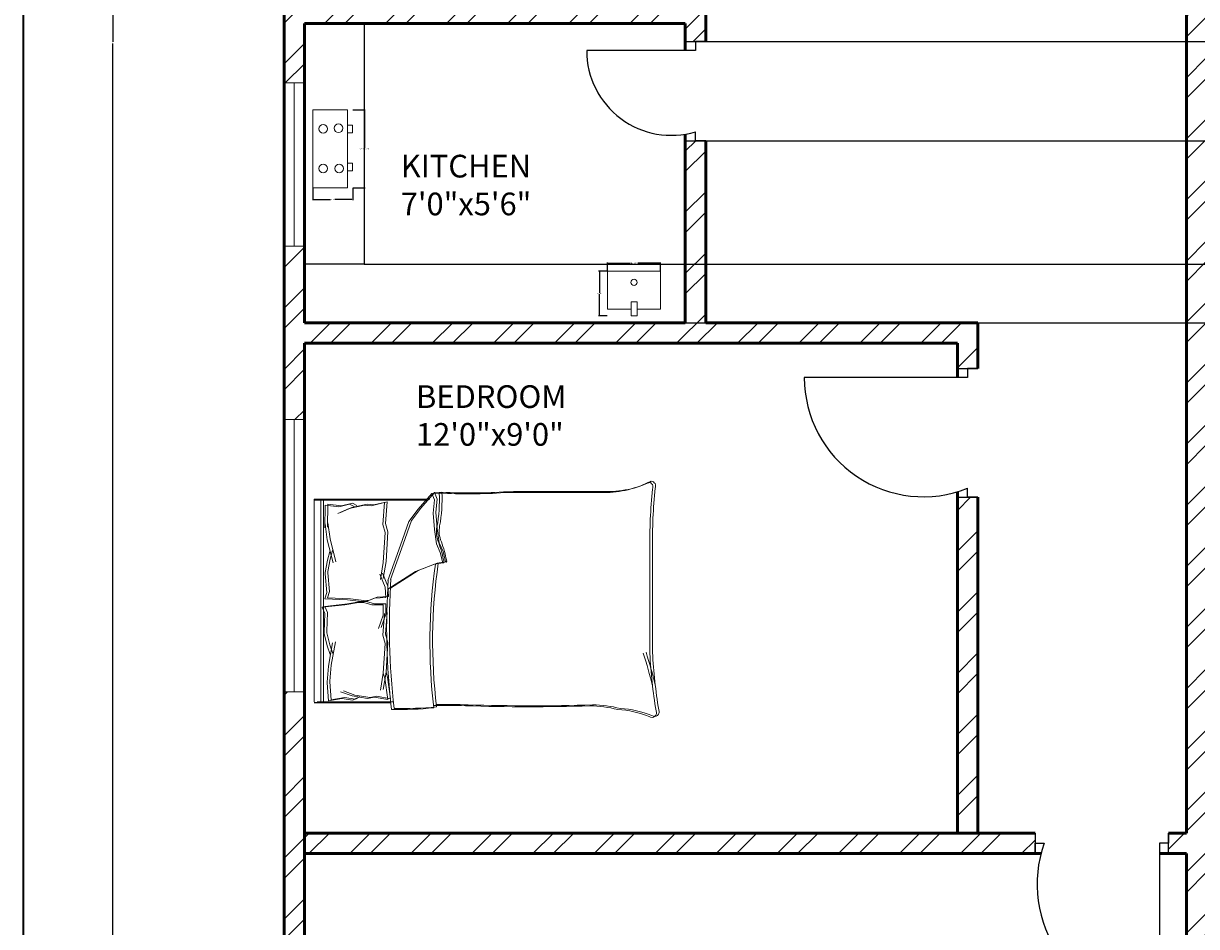
# Model space of a CAD drawing. Units: inches. Extents: x 2129 to 2642, y 1542 to 2414.
# Tile 2 of 9: x 2129 to 2388, y 1808 to 2007. Entities that reach past the tile are written whole.
import ezdxf

# ---------------------------------------------------------------- set-up
doc = ezdxf.new("R2010")
doc.units = ezdxf.units.IN
for name, color, linetype, lineweight in [('A-ANNO-DIMS', 2, 'Continuous', 18), ('A-ANNO-TTLB', 7, 'Continuous', 35), ('A-AREA-IDEN', 7, 'Continuous', 18), ('A-DOOR', 3, 'Continuous', 25), ('A-EQPM', 8, 'Continuous', 18), ('A-FLOR-CASE', 8, 'Continuous', 25), ('A-FLOR-FIXT', 9, 'Continuous', 18), ('A-FURN', 8, 'Continuous', 18), ('A-GLAZ', 4, 'Continuous', 18), ('A-WALL', 7, 'Continuous', 50), ('A-WALL-PATT', 252, 'Continuous', 13)]:
    doc.layers.add(name, color=color, linetype=linetype, lineweight=lineweight)
doc.styles.get("Standard").update_dxf_attribs({"font": 'arial.ttf'})
doc.dimstyles.get("Standard").update_dxf_attribs({"dimtxt": 0.18, "dimasz": 0.18, "dimexe": 0.18, "dimexo": 0.0625, "dimgap": 0.09, "dimtad": 0, "dimtih": 1, "dimtoh": 1, "dimdec": 4, "dimzin": 0, "dimdsep": 46, "dimtxsty": 'Standard', "dimcen": 0.09, "dimadec": 0, "dimazin": 0, "dimtfac": 1, "dimtdec": 4, "dimtofl": 0, "dimtmove": 0, "dimatfit": 3, "dimfxl": 1, "dimtolj": 1, "dimtzin": 0, "dimarcsym": 0})

# ---------------------------------------------------------------- blocks, each defined once
blk = doc.blocks.new('BED-DOUBLE')
for p, q in [((3.24, 59.14), (3.24, 76.05)), ((3.25, 59.14), (3.25, 76.05)), ((48.08, 76.05), (3.46, 76.05)), ((3.46, 58.54), (3.46, 75.45)), ((3.46, 58.54), (3.46, 75.45)), ((47.87, 76.05), (47.87, 51.2)), ((47.87, 76.05), (47.87, 51.2)), ((48.08, 76.05), (48.08, 75.45)), ((48.08, 75.45), (48.08, 50.6)), ((48.08, 75.45), (48.08, 50.6)), ((3.24, 74.61), (47.87, 74.61)), ((3.25, 74.61), (47.87, 74.61)), ((3.46, 74.02), (48.08, 74.02)), ((3.46, 74.02), (48.08, 74.02)), ((3.64, 72.93), (7.64, 73.24)), ((3.64, 72.93), (7.64, 73.24)), ((3.64, 72.95), (4.18, 69.98)), ((3.64, 72.95), (4.18, 69.98)), ((3.85, 72.33), (7.85, 72.64)), ((3.85, 72.33), (7.85, 72.64)), ((7.64, 73.24), (7.74, 73.22)), ((7.64, 73.24), (7.74, 73.22)), ((7.74, 73.22), (11.31, 72.95)), ((7.74, 73.22), (11.31, 72.95)), ((7.85, 72.64), (7.95, 72.62)), ((7.85, 72.64), (7.95, 72.62)), ((7.95, 72.62), (11.52, 72.35)), ((7.95, 72.62), (11.52, 72.35)), ((11.31, 72.95), (16.44, 72.01)), ((11.31, 72.95), (16.44, 72.01)), ((13.87, 72.55), (15.76, 73.22)), ((13.87, 72.55), (15.76, 73.22)), ((14.08, 71.95), (15.97, 72.62)), ((14.08, 71.95), (15.97, 72.62)), ((15.76, 73.22), (18.46, 73.9)), ((15.76, 73.22), (18.46, 73.9)), ((15.97, 72.62), (18.67, 73.3)), ((15.97, 72.62), (18.67, 73.3)), ((18.46, 73.9), (18.76, 73.9)), ((18.46, 73.9), (18.76, 73.9)), ((18.67, 73.3), (18.97, 73.3)), ((18.67, 73.3), (18.97, 73.3)), ((18.76, 73.9), (22.91, 73.76)), ((18.76, 73.9), (22.91, 73.76)), ((18.97, 73.3), (23.12, 73.16)), ((18.97, 73.3), (23.12, 73.16)), ((22.91, 73.76), (24.26, 74.3)), ((22.91, 73.76), (24.26, 74.3)), ((23.12, 73.16), (24.47, 73.7)), ((23.12, 73.16), (24.47, 73.7)), ((24.26, 74.3), (24.8, 69.31)), ((24.26, 74.3), (24.8, 69.31)), ((24.47, 73.7), (25.01, 68.71)), ((24.47, 73.7), (25.01, 68.71)), ((26.12, 73.72), (25.9, 68.7)), ((26.12, 73.72), (25.9, 68.7)), ((26.34, 73.12), (26.11, 68.1)), ((26.34, 73.12), (26.11, 68.1)), ((27.5, 73.27), (26.12, 73.72)), ((27.5, 73.27), (26.12, 73.72)), ((27.72, 72.67), (26.34, 73.12)), ((27.72, 72.67), (26.34, 73.12)), ((31.64, 73.66), (27.5, 73.27)), ((31.64, 73.66), (27.5, 73.27)), ((31.85, 73.06), (27.72, 72.67)), ((31.85, 73.06), (27.72, 72.67)), ((31.94, 73.68), (31.64, 73.66)), ((31.94, 73.68), (31.64, 73.66)), ((32.15, 73.08), (31.85, 73.06)), ((32.15, 73.08), (31.85, 73.06)), ((34.68, 73.17), (31.94, 73.68)), ((34.67, 73.17), (31.94, 73.68)), ((34.89, 72.58), (32.15, 73.08)), ((34.89, 72.58), (32.15, 73.08)), ((39.14, 73.18), (34.08, 71.92)), ((39.14, 73.18), (34.08, 71.92)), ((39.35, 72.58), (34.29, 71.32)), ((39.35, 72.58), (34.29, 71.32)), ((36.6, 72.62), (34.67, 73.17)), ((36.6, 72.62), (34.68, 73.17)), ((36.82, 72.02), (34.89, 72.58)), ((36.82, 72.02), (34.89, 72.58)), ((42.68, 73.67), (39.14, 73.18)), ((42.68, 73.67), (39.14, 73.18)), ((42.9, 73.08), (39.35, 72.58)), ((42.9, 73.08), (39.35, 72.58)), ((46.79, 73.66), (41.75, 73.75)), ((41.75, 73.75), (42.68, 73.67)), ((46.79, 73.66), (41.75, 73.75)), ((41.75, 73.75), (42.68, 73.67)), ((47.01, 73.06), (41.96, 73.15)), ((41.96, 73.15), (42.9, 73.08)), ((47.01, 73.06), (41.96, 73.15)), ((41.96, 73.15), (42.9, 73.08)), ((46.79, 73.66), (46.44, 70.66)), ((46.79, 73.66), (46.44, 70.66)), ((47.01, 73.06), (46.65, 70.06)), ((47.01, 73.06), (46.65, 70.06)), ((4.18, 69.98), (3.77, 67.55)), ((4.18, 69.98), (3.77, 67.55)), ((3.85, 72.35), (4.39, 69.38)), ((3.85, 72.35), (4.39, 69.38)), ((4.72, 67.69), (5.66, 70.25)), ((4.72, 67.69), (5.66, 70.25)), ((11.52, 72.35), (16.65, 71.41)), ((11.52, 72.35), (16.65, 71.41)), ((46.04, 68.34), (44.94, 70.84)), ((46.04, 68.34), (44.94, 70.84)), ((46.26, 67.74), (45.15, 70.24)), ((46.26, 67.74), (45.15, 70.24)), ((46.44, 70.66), (46.99, 68.26)), ((46.44, 70.66), (46.99, 68.26)), ((46.65, 70.06), (47.21, 67.66)), ((46.65, 70.06), (47.21, 67.66)), ((3.77, 67.55), (4.31, 66.61)), ((3.77, 67.55), (4.31, 66.61)), ((4.39, 69.38), (3.98, 66.95)), ((4.39, 69.38), (3.99, 66.95)), ((4.18, 64.31), (4.72, 67.69)), ((4.18, 64.31), (4.72, 67.69)), ((4.93, 67.09), (5.87, 69.65)), ((4.93, 67.09), (5.87, 69.65)), ((24.8, 69.31), (25.34, 66.34)), ((24.8, 69.31), (25.34, 66.34)), ((25.01, 68.71), (25.55, 65.74)), ((25.01, 68.71), (25.55, 65.74)), ((25.9, 68.7), (25.54, 65.7)), ((25.9, 68.7), (25.54, 65.7)), ((26.11, 68.1), (25.76, 65.11)), ((26.11, 68.1), (25.76, 65.11)), ((46.79, 65), (46.04, 68.34)), ((46.79, 65), (46.04, 68.34)), ((47.01, 64.41), (46.26, 67.74)), ((47.01, 64.41), (46.26, 67.74)), ((46.99, 68.26), (46.51, 67.28)), ((46.99, 68.26), (46.51, 67.28)), ((47.21, 67.66), (46.73, 66.69)), ((47.21, 67.66), (46.73, 66.69)), ((3.98, 66.95), (4.52, 66.01)), ((3.99, 66.95), (4.53, 66.01)), ((4.39, 63.71), (4.93, 67.09)), ((4.39, 63.71), (4.93, 67.09)), ((25.34, 65.12), (24.8, 63.36)), ((25.34, 65.12), (24.8, 63.36)), ((25.34, 66.34), (25.34, 65.12)), ((25.34, 66.34), (25.34, 65.12)), ((25.54, 65.7), (25.62, 64.49)), ((25.54, 65.7), (25.62, 64.49)), ((25.55, 65.74), (25.55, 64.52)), ((25.55, 65.74), (25.55, 64.52)), ((25.76, 65.11), (25.83, 63.89)), ((25.76, 65.11), (25.83, 63.89)), ((46.62, 63.5), (46.79, 65)), ((46.62, 63.5), (46.79, 65)), ((3.91, 59.85), (4.45, 62.82)), ((3.91, 59.85), (4.45, 62.82)), ((4.12, 59.26), (4.66, 62.23)), ((4.12, 59.26), (4.66, 62.23)), ((4.45, 62.82), (4.18, 64.31)), ((4.45, 62.82), (4.18, 64.31)), ((4.66, 62.23), (4.39, 63.71)), ((4.66, 62.23), (4.39, 63.71)), ((24.8, 63.36), (24.8, 60.86)), ((24.8, 63.36), (24.8, 60.86)), ((25.55, 64.52), (25.01, 62.77)), ((25.55, 64.52), (25.01, 62.77)), ((25.01, 62.77), (25.01, 60.26)), ((25.01, 62.77), (25.01, 60.26)), ((25.62, 64.49), (26.27, 62.77)), ((25.62, 64.49), (26.27, 62.77)), ((25.83, 63.89), (26.48, 62.18)), ((25.83, 63.89), (26.48, 62.18)), ((26.27, 62.77), (26.42, 60.27)), ((26.27, 62.77), (26.42, 60.27)), ((26.48, 62.18), (26.64, 59.68)), ((26.48, 62.18), (26.64, 59.68)), ((47.34, 60.57), (46.62, 63.5)), ((47.34, 60.57), (46.62, 63.5)), ((46.83, 62.91), (47.01, 64.41)), ((46.83, 62.91), (47.01, 64.41)), ((47.55, 59.98), (46.83, 62.91)), ((47.55, 59.98), (46.83, 62.91)), ((8.67, 60.53), (3.91, 59.85)), ((8.67, 60.53), (3.91, 59.85)), ((8.88, 59.93), (4.12, 59.26)), ((8.88, 59.93), (4.12, 59.26)), ((5.96, 61.45), (9.72, 60.83)), ((5.96, 61.45), (9.72, 60.83)), ((6.17, 60.86), (9.94, 60.23)), ((6.17, 60.86), (9.94, 60.23)), ((9.72, 60.83), (8.67, 60.53)), ((9.72, 60.83), (8.67, 60.53)), ((9.94, 60.23), (8.88, 59.93)), ((9.94, 60.23), (8.88, 59.93)), ((9.72, 60.83), (16.27, 60.43)), ((9.72, 60.83), (16.27, 60.43)), ((9.94, 60.23), (16.48, 59.83)), ((9.94, 60.23), (16.48, 59.83)), ((16.27, 60.43), (18.1, 60.95)), ((16.27, 60.43), (18.1, 60.95)), ((16.48, 59.83), (18.31, 60.35)), ((16.48, 59.83), (18.31, 60.35)), ((18.1, 60.95), (22.89, 60.57)), ((18.1, 60.95), (22.89, 60.57)), ((18.31, 60.35), (23.11, 59.98)), ((18.31, 60.35), (23.1, 59.98)), ((22.51, 60.86), (19.57, 61.88)), ((22.51, 60.86), (19.57, 61.88)), ((22.72, 60.26), (19.78, 61.28)), ((22.72, 60.26), (19.78, 61.28)), ((24.8, 60.86), (22.51, 60.86)), ((24.8, 60.86), (22.51, 60.86)), ((25.01, 60.26), (22.72, 60.26)), ((25.01, 60.26), (22.72, 60.26)), ((26.42, 60.27), (28.71, 60.42)), ((26.42, 60.27), (28.71, 60.42)), ((26.64, 59.68), (28.93, 59.82)), ((26.64, 59.68), (28.93, 59.82)), ((28.25, 59.82), (32.17, 53.75)), ((28.25, 59.82), (32.17, 53.75)), ((28.71, 60.42), (31.58, 61.62)), ((28.71, 60.42), (31.58, 61.62)), ((28.93, 59.82), (31.79, 61.02)), ((28.93, 59.82), (31.79, 61.02)), ((37.95, 57.08), (30.17, 59.82)), ((37.95, 57.08), (30.17, 59.82)), ((30.41, 61.45), (34.17, 60.83)), ((30.41, 61.45), (34.17, 60.83)), ((30.62, 60.86), (34.39, 60.23)), ((30.62, 60.86), (34.38, 60.23)), ((34.17, 60.83), (40.72, 60.43)), ((34.17, 60.83), (40.72, 60.43)), ((34.38, 60.23), (40.93, 59.83)), ((34.39, 60.23), (40.93, 59.83)), ((40.72, 60.43), (42.55, 60.95)), ((40.72, 60.43), (42.55, 60.95)), ((40.93, 59.83), (42.76, 60.35)), ((40.93, 59.83), (42.76, 60.35)), ((42.55, 60.95), (47.34, 60.57)), ((42.55, 60.95), (47.34, 60.57)), ((42.76, 60.35), (47.55, 59.98)), ((42.76, 60.35), (47.55, 59.98)), ((28.47, 59.22), (32.38, 53.16)), ((28.47, 59.22), (32.38, 53.16)), ((38.16, 56.48), (30.38, 59.22)), ((38.16, 56.48), (30.38, 59.22)), ((43.16, 55.2), (37.95, 57.08)), ((43.16, 55.2), (37.95, 57.08)), ((43.37, 54.6), (38.16, 56.48)), ((43.37, 54.6), (38.16, 56.48)), ((45.91, 53.17), (43.16, 55.2)), ((45.91, 53.17), (43.16, 55.2)), ((46.12, 52.58), (43.37, 54.6)), ((46.12, 52.58), (43.37, 54.6)), ((32.17, 53.75), (33.76, 49.56)), ((32.17, 53.75), (33.76, 49.56)), ((32.38, 53.16), (33.97, 48.96)), ((32.38, 53.16), (33.97, 48.96)), ((49.37, 50.14), (45.91, 53.17)), ((49.36, 50.14), (45.91, 53.17)), ((49.58, 49.54), (46.12, 52.58)), ((49.58, 49.54), (46.12, 52.58)), ((33.76, 49.56), (34.05, 47.68)), ((33.76, 49.56), (34.05, 47.68)), ((38.24, 49.13), (41.42, 49.56)), ((38.24, 49.13), (41.42, 49.56)), ((41.42, 49.56), (45.04, 49.85)), ((41.42, 49.56), (45.04, 49.85)), ((41.64, 48.96), (45.25, 49.25)), ((41.64, 48.96), (45.25, 49.25)), ((45.04, 49.85), (47.93, 49.56)), ((45.04, 49.85), (47.93, 49.56)), ((45.25, 49.25), (48.14, 48.96)), ((45.25, 49.25), (48.14, 48.96)), ((47.93, 49.56), (49.37, 50.14)), ((47.93, 49.56), (49.36, 50.14)), ((48.14, 48.96), (49.58, 49.54)), ((48.14, 48.96), (49.58, 49.54)), ((49.44, 48.51), (49.36, 50.14, 3.61)), ((49.44, 48.51), (49.37, 50.14, 3.61)), ((49.65, 47.91), (49.58, 49.54, 3.61)), ((49.65, 47.91), (49.58, 49.54, 3.61)), ((33.97, 48.96), (34.26, 47.09)), ((33.97, 48.96), (34.26, 47.09)), ((34.05, 47.68), (36.36, 48.26)), ((34.05, 47.68), (36.36, 48.26)), ((34.26, 47.09), (36.57, 47.66)), ((34.26, 47.09), (36.57, 47.66)), ((36.36, 48.26), (38.24, 49.13)), ((36.36, 48.26), (38.24, 49.13)), ((36.57, 47.66), (38.45, 48.53)), ((36.57, 47.66), (38.45, 48.53)), ((38.45, 48.53), (41.64, 48.96)), ((38.45, 48.53), (41.64, 48.96)), ((14.07, 2.05), (37.05, 2.05)), ((14.07, 2.05), (37.05, 2.05)), ((14.28, 1.46), (37.26, 1.46)), ((14.28, 1.46), (37.26, 1.46))]:
    blk.add_line(p, q)
for centre, radius, start, end in [((19.94, -93.94), 154.04, 86.0865, 96.7821), ((19.94, -93.94), 154.04, 86.0865, 96.7821), ((79.52, 57.28), 77.79, 178.7218, 185.604), ((79.52, 57.28), 77.79, 178.7218, 185.604), ((79.73, 56.69), 77.79, 178.7218, 185.604), ((79.73, 56.69), 77.79, 178.7218, 185.604), ((20.16, -94.54), 154.04, 86.0865, 96.7821), ((20.16, -94.54), 154.04, 86.0865, 96.7821), ((16.58, -69.91), 120.47, 81.7845, 96.9006), ((16.58, -69.91), 120.47, 81.7845, 96.9006), ((16.79, -70.51), 120.47, 81.7845, 96.9006), ((16.79, -70.51), 120.47, 81.7845, 96.9006), ((-156.22, 46.94), 158.84, 358.4762, 1.0082), ((-156.22, 46.94), 158.84, 358.4762, 1.0082), ((-156.01, 46.34), 158.84, 358.4762, 1.0082), ((-156.01, 46.34), 158.84, 358.4762, 1.0082), ((34.21, 47.62), 0.172, 160.2464, 271.1377), ((34.21, 47.62), 0.172, 160.2464, 271.1377), ((29.09, 74.66), 27.69, 280.6617, 289.8806), ((29.09, 74.66), 27.69, 280.6617, 289.8806), ((34.42, 47.03), 0.172, 160.2464, 271.1377), ((34.42, 47.03), 0.172, 160.2464, 271.1377), ((29.3, 74.07), 27.69, 280.6617, 289.8806), ((29.3, 74.07), 27.69, 280.6617, 289.8806), ((40.85, 43.3), 5.81, 78.6608, 113.7384), ((40.85, 43.3), 5.81, 78.6608, 113.7384), ((41.06, 42.71), 5.81, 78.6608, 113.7384), ((41.06, 42.71), 5.81, 78.6608, 113.7384), ((47.93, 82.26), 33.79, 259.8763, 272.5657), ((47.93, 82.26), 33.79, 259.8763, 272.5657), ((48.14, 81.67), 33.79, 259.8763, 272.5657), ((48.14, 81.67), 33.79, 259.8763, 272.5657), ((170.19, 42.14), 120.92, 176.9791, 183.8365), ((170.19, 42.14), 120.92, 176.9791, 183.8365), ((170.4, 41.54), 120.92, 176.9791, 183.8365), ((170.4, 41.54), 120.92, 176.9791, 183.8365), ((452.7, 28.79), 450.36, 178.2277, 181.7185), ((452.7, 28.79), 450.36, 178.2277, 181.7185), ((452.91, 28.19), 450.36, 178.2277, 181.7185), ((452.91, 28.19), 450.36, 178.2277, 181.7185), ((-4210.02, 12.72), 4259.62, 0.00217, 0.28689), ((-4210.02, 12.72), 4259.62, 0.00217, 0.28689), ((-4209.81, 12.12), 4259.62, 0.00217, 0.28689), ((-4209.81, 12.12), 4259.62, 0.00217, 0.28689), ((-25.12, 15.81), 27.67, 346.0648, 358.9113), ((-25.12, 15.81), 27.67, 346.0648, 358.9113), ((-24.9, 15.21), 27.67, 346.0648, 358.9113), ((-24.9, 15.21), 27.67, 346.0648, 358.9113), ((71.11, 11.93), 21.54, 177.4714, 206.4681), ((71.11, 11.93), 21.54, 177.4714, 206.4681), ((71.33, 11.33), 21.54, 177.4714, 206.4681), ((71.32, 11.33), 21.54, 177.4714, 206.4681), ((-20.22, 10.43), 22, 337.9751, 356.652), ((-20.22, 10.43), 22, 337.9751, 356.652), ((-20.01, 9.83), 22, 337.9751, 356.652), ((-20.01, 9.83), 22, 337.9751, 356.652), ((-16.08, 98.19), 99.41, 283.3832, 287.7053), ((-16.08, 98.19), 99.41, 283.3832, 287.7053), ((-15.87, 97.59), 99.41, 283.3832, 287.7053), ((-15.87, 97.59), 99.41, 283.3832, 287.7053), ((1.02, 1.61), 1.02, 146.1736, 293.4781), ((1.02, 1.61), 1.02, 146.1736, 293.4781), ((1.23, 1.01), 1.02, 146.1736, 293.4781), ((1.23, 1.01), 1.02, 146.1736, 293.4781), ((20.01, -111.48), 113.69, 92.9958, 99.4091), ((20.01, -111.48), 113.69, 92.9958, 99.4091), ((20.22, -112.08), 113.69, 92.9958, 99.4091), ((20.22, -112.08), 113.69, 92.9958, 99.4091), ((38.43, -122.17), 124.23, 84.4998, 90.6351), ((38.43, -122.17), 124.23, 84.4998, 90.6351), ((38.64, -122.76), 124.23, 84.4998, 90.6351), ((38.64, -122.76), 124.23, 84.4998, 90.6351), ((50.81, 2.4), 1.03, 242.6588, 356.02), ((50.81, 2.4), 1.03, 242.6588, 356.02), ((51.02, 1.81), 1.03, 242.6588, 356.02), ((51.02, 1.81), 1.03, 242.6588, 356.02)]:
    blk.add_arc(centre, radius, start, end)
blk = doc.blocks.new('COOKTOP-4-BURNER')
for points in [[(0, 17.17), (7.64, 17.17), (7.64, 0), (0, 0)], [(7.64, 13.8), (8.8, 13.8), (8.8, 12.1), (7.64, 12.1)], [(7.64, 5.39), (8.8, 5.39), (8.8, 3.7), (7.64, 3.7)]]:
    blk.add_lwpolyline(points, close=True)
for centre in [(2.31, 13.01), (5.67, 13.11), (2.31, 4.27), (5.8, 4.27)]:
    blk.add_circle(centre, 0.951)
blk = doc.blocks.new('SINK-KITCHEN')
blk.add_lwpolyline([(5.28, 1.49), (0, 1.49), (0, 9.84), (11.71, 9.84), (11.71, 1.49), (6.54, 1.49)])
blk.add_lwpolyline([(5.28, 3.09), (6.54, 3.09), (6.54, 0), (5.28, 0)], close=True)
blk.add_circle((5.88, 7.38), 0.679)
blk = doc.blocks.new('WIN-60-B')
for p, q in [((4.5, 60), (0, 60)), ((0, 60), (2.25, 60)), ((2.25, 60), (2.25, 0)), ((2.25, 0), (0, 0)), ((0, 0), (4.5, 0))]:
    blk.add_line(p, q)
blk = doc.blocks.new('WIN-36')
for p, q in [((4.5, 36), (0, 36)), ((0, 36), (2.25, 36)), ((2.25, 36), (2.25, 0)), ((4.5, 0), (0, 0)), ((2.25, 0), (4.5, 0))]:
    blk.add_line(p, q)
blk = doc.blocks.new('*D28')
at = {"layer": 'A-ANNO-DIMS', "color": 0, "lineweight": -2, "transparency": 16777216}
for p, q in [((2202.11, 1988.17), (2204.8, 1988.17)), ((2204.62, 1987.99), (2204.62, 1979.77)), ((2204.62, 1971.18), (2204.62, 1979.4)), ((2202.11, 1971), (2204.8, 1971))]:
    blk.add_line(p, q, dxfattribs=at)
at = {"layer": 'A-ANNO-DIMS', "color": 0, "transparency": 16777216}
for points in [[(2204.59, 1987.99), (2204.65, 1987.99), (2204.62, 1988.17)], [(2204.59, 1971.18), (2204.65, 1971.18), (2204.62, 1971)]]:
    blk.add_solid(points, dxfattribs=at)
at = {"layer": 'Defpoints', "color": 0, "transparency": 16777216}
for p in [(2202.05, 1988.17), (2204.62, 1988.17), (2202.05, 1971)]:
    blk.add_point(p, dxfattribs=at)
at = {"layer": 'A-ANNO-DIMS', "color": 0, "transparency": 16777216, "insert": (2204.62, 1979.59), "char_height": 0.18, "attachment_point": 5}
blk.add_mtext('\\A1;COOKTOP 17 TYP.', dxfattribs=at)
blk = doc.blocks.new('*D29')
at = {"layer": 'A-ANNO-DIMS', "color": 0, "lineweight": -2, "transparency": 16777216}
for p, q in [((2193.24, 1970.94), (2193.24, 1968.24)), ((2202.05, 1970.94), (2202.05, 1968.24)), ((2193.42, 1968.42), (2197.19, 1968.42)), ((2201.87, 1968.42), (2198.1, 1968.42))]:
    blk.add_line(p, q, dxfattribs=at)
at = {"layer": 'A-ANNO-DIMS', "color": 0, "transparency": 16777216}
for points in [[(2193.42, 1968.45), (2193.42, 1968.39), (2193.24, 1968.42)], [(2201.87, 1968.45), (2201.87, 1968.39), (2202.05, 1968.42)]]:
    blk.add_solid(points, dxfattribs=at)
at = {"layer": 'Defpoints', "color": 0, "transparency": 16777216}
for p in [(2193.24, 1971), (2202.05, 1971), (2202.05, 1968.42)]:
    blk.add_point(p, dxfattribs=at)
at = {"layer": 'A-ANNO-DIMS', "color": 0, "transparency": 16777216, "insert": (2197.64, 1968.42), "char_height": 0.18, "attachment_point": 5}
blk.add_mtext('\\A1;9 TYP.', dxfattribs=at)
blk = doc.blocks.new('*D30')
at = {"layer": 'A-ANNO-DIMS', "color": 0, "lineweight": -2, "transparency": 16777216}
for p, q in [((2258.22, 1952.68), (2258.22, 1954.55)), ((2258.4, 1954.37), (2263.21, 1954.37)), ((2269.74, 1954.37), (2264.93, 1954.37)), ((2269.92, 1952.68), (2269.92, 1954.55))]:
    blk.add_line(p, q, dxfattribs=at)
at = {"layer": 'A-ANNO-DIMS', "color": 0, "transparency": 16777216}
for points in [[(2258.4, 1954.4), (2258.4, 1954.34), (2258.22, 1954.37)], [(2269.74, 1954.4), (2269.74, 1954.34), (2269.92, 1954.37)]]:
    blk.add_solid(points, dxfattribs=at)
at = {"layer": 'Defpoints', "color": 0, "transparency": 16777216}
for p in [(2269.92, 1954.37), (2258.22, 1952.61), (2269.92, 1952.61)]:
    blk.add_point(p, dxfattribs=at)
at = {"layer": 'A-ANNO-DIMS', "color": 0, "transparency": 16777216, "insert": (2264.07, 1954.37), "char_height": 0.18, "attachment_point": 5}
blk.add_mtext('\\A1;SINK 12 TYP.', dxfattribs=at)
blk = doc.blocks.new('*D31')
at = {"layer": 'A-ANNO-DIMS', "color": 0, "lineweight": -2, "transparency": 16777216}
for p, q in [((2258.15, 1952.61), (2256.28, 1952.61)), ((2256.46, 1952.43), (2256.46, 1947.87)), ((2256.46, 1942.95), (2256.46, 1947.51)), ((2258.15, 1942.77), (2256.28, 1942.77))]:
    blk.add_line(p, q, dxfattribs=at)
at = {"layer": 'A-ANNO-DIMS', "color": 0, "transparency": 16777216}
for points in [[(2256.43, 1952.43), (2256.49, 1952.43), (2256.46, 1952.61)], [(2256.43, 1942.95), (2256.49, 1942.95), (2256.46, 1942.77)]]:
    blk.add_solid(points, dxfattribs=at)
at = {"layer": 'Defpoints', "color": 0, "transparency": 16777216}
for p in [(2256.46, 1952.61), (2258.22, 1952.61), (2258.22, 1942.77)]:
    blk.add_point(p, dxfattribs=at)
at = {"layer": 'A-ANNO-DIMS', "color": 0, "transparency": 16777216, "insert": (2256.46, 1947.69), "char_height": 0.18, "attachment_point": 5}
blk.add_mtext('\\A1;10 TYP.', dxfattribs=at)
blk = doc.blocks.new('*D35')
at = {"layer": 'A-ANNO-DIMS', "color": 0, "lineweight": -2, "transparency": 16777216}
for p, q in [((2186.84, 2340.22), (2148.97, 2340.22)), ((2149.15, 2340.04), (2149.15, 2003.15)), ((2149.15, 1665.9), (2149.15, 2002.79)), ((2186.84, 1665.72), (2148.97, 1665.72))]:
    blk.add_line(p, q, dxfattribs=at)
at = {"layer": 'A-ANNO-DIMS', "color": 0, "transparency": 16777216}
for points in [[(2149.12, 2340.04), (2149.18, 2340.04), (2149.15, 2340.22)], [(2149.12, 1665.9), (2149.18, 1665.9), (2149.15, 1665.72)]]:
    blk.add_solid(points, dxfattribs=at)
at = {"layer": 'Defpoints', "color": 0, "transparency": 16777216}
for p in [(2149.15, 2340.22), (2186.9, 2340.22), (2186.9, 1665.72)]:
    blk.add_point(p, dxfattribs=at)
at = {"layer": 'A-ANNO-DIMS', "color": 0, "transparency": 16777216, "insert": (2149.15, 2002.97), "char_height": 0.18, "attachment_point": 5}
blk.add_mtext('\\A1;674.5', dxfattribs=at)
blk = doc.blocks.new('*D47')
at = {"layer": 'A-ANNO-DIMS', "color": 0, "lineweight": -2, "transparency": 16777216}
for p, q in [((2279.97, 2003.23), (2626.83, 2003.23)), ((2626.65, 2003.05), (2626.65, 1992.47)), ((2626.65, 1981.52), (2626.65, 1992.1)), ((2279.97, 1981.34), (2626.83, 1981.34))]:
    blk.add_line(p, q, dxfattribs=at)
at = {"layer": 'A-ANNO-DIMS', "color": 0, "transparency": 16777216}
for points in [[(2626.62, 2003.05), (2626.68, 2003.05), (2626.65, 2003.23)], [(2626.62, 1981.52), (2626.68, 1981.52), (2626.65, 1981.34)]]:
    blk.add_solid(points, dxfattribs=at)
at = {"layer": 'Defpoints', "color": 0, "transparency": 16777216}
for p in [(2279.9, 2003.23), (2626.65, 2003.23), (2279.9, 1981.34)]:
    blk.add_point(p, dxfattribs=at)
at = {"layer": 'A-ANNO-DIMS', "color": 0, "transparency": 16777216, "insert": (2626.65, 1992.29), "char_height": 0.18, "attachment_point": 5}
blk.add_mtext('\\A1;21.886', dxfattribs=at)
blk = doc.blocks.new('*D49')
at = {"layer": 'A-ANNO-DIMS', "color": 0, "lineweight": -2, "transparency": 16777216}
for p, q in [((2275.47, 1954.17), (2626.83, 1954.17)), ((2626.65, 1953.99), (2626.65, 1947.88)), ((2626.65, 1941.4), (2626.65, 1947.52)), ((2275.47, 1941.22), (2626.83, 1941.22))]:
    blk.add_line(p, q, dxfattribs=at)
at = {"layer": 'A-ANNO-DIMS', "color": 0, "transparency": 16777216}
for points in [[(2626.62, 1953.99), (2626.68, 1953.99), (2626.65, 1954.17)], [(2626.62, 1941.4), (2626.68, 1941.4), (2626.65, 1941.22)]]:
    blk.add_solid(points, dxfattribs=at)
at = {"layer": 'Defpoints', "color": 0, "transparency": 16777216}
for p in [(2275.4, 1954.17), (2626.65, 1954.17), (2275.4, 1941.22)]:
    blk.add_point(p, dxfattribs=at)
at = {"layer": 'A-ANNO-DIMS', "color": 0, "transparency": 16777216, "insert": (2626.65, 1947.7), "char_height": 0.18, "attachment_point": 5}
blk.add_mtext('\\A1;12.953', dxfattribs=at)

msp = doc.modelspace()

# ---------------------------------------------------------------- hatches: boundary and pattern name
at = {"layer": 'A-WALL-PATT'}
h = msp.add_hatch(dxfattribs=at)
h.set_pattern_fill('ANSI32', color=256)
h.paths.add_polyline_path([(2306.2606, 2305.9717), (2306.2606, 2308.2217), (2276.3515, 2308.2217), (2276.3515, 2303.7217), (2306.2606, 2303.7217)])
h.paths.add_polyline_path([(2216.3515, 2305.9717), (2216.3515, 2308.2217), (2186.9043, 2308.2217), (2186.9043, 2278.1696), (2191.4043, 2278.1696), (2191.4043, 2303.7217), (2216.3515, 2303.7217)])
h.paths.add_polyline_path([(2339.9043, 2335.7217), (2362.1938, 2335.7217), (2362.1938, 2340.2217), (2335.4043, 2340.2217), (2335.4043, 2308.2217), (2329.3487, 2308.2217), (2329.3487, 2305.9717), (2329.3487, 2303.7217), (2335.4043, 2303.7217), (2335.4043, 2186.7217), (2329.4345, 2186.7217), (2329.4345, 2182.2217), (2335.4043, 2182.2217), (2335.4043, 2174.7178), (2339.9043, 2174.7178), (2339.9043, 2182.2217), (2339.9043, 2303.7217)])
h.paths.add_polyline_path([(2440.4043, 2340.2217), (2411.654, 2340.2217), (2411.654, 2335.7217), (2435.9043, 2335.7217), (2435.9043, 2303.7217), (2435.9043, 2182.2217), (2435.9043, 2174.1935), (2438.1543, 2174.1935), (2440.4043, 2174.1935), (2440.4043, 2182.2217), (2444.653, 2182.2217), (2444.653, 2184.4717), (2444.653, 2186.7217), (2440.4043, 2186.7217), (2440.4043, 2303.7217), (2445.8547, 2303.7217), (2445.8547, 2308.2217), (2440.4043, 2308.2217)])
h.paths.add_polyline_path([(2498.2381, 2308.2217), (2470.3901, 2308.2217), (2470.3901, 2303.7217), (2498.2381, 2303.7217), (2498.2381, 2305.9717)])
h.paths.add_polyline_path([(2588.9043, 2308.2217), (2586.9043, 2308.2217), (2558.2381, 2308.2217), (2558.2381, 2303.7217), (2584.4043, 2303.7217), (2584.4043, 2279.1087), (2588.9043, 2279.1087)])
h.paths.add_polyline_path([(2588.9043, 2219.1087), (2584.4043, 2219.1087), (2584.4043, 2186.7217), (2478.0667, 2186.7217), (2478.0667, 2182.2217), (2584.4043, 2182.2217), (2584.4043, 2157.7883), (2588.9043, 2157.7883)])
h.paths.add_polyline_path([(2588.9043, 2097.7883), (2584.6063, 2097.7883), (2584.6063, 2075.5462, -0.09241561), (2584.4043, 2074.4627), (2584.4043, 2064.2217), (2495.9043, 2064.2217), (2495.9043, 2040.4611), (2500.4043, 2040.4611), (2500.4043, 2059.7217), (2584.4043, 2059.7217), (2584.4043, 2052.2164), (2588.9043, 2052.2164)])
h.paths.add_polyline_path([(2588.9043, 2028.2164), (2584.4043, 2028.2164), (2584.4043, 2011.7217), (2500.4043, 2011.7217), (2500.4043, 2015.243), (2498.1543, 2015.243), (2495.9043, 2015.243), (2495.9043, 2007.2217), (2495.9043, 2003.7597), (2500.4043, 2003.7597), (2500.4043, 2007.2217), (2584.4043, 2007.2217), (2584.4043, 1992.1997), (2588.9043, 1992.1997)])
h.paths.add_polyline_path([(2588.9043, 1956.1997), (2584.4043, 1956.1997), (2584.4043, 1941.2217), (2500.4043, 1941.2217), (2500.4043, 1985.1493), (2498.1543, 1985.1493), (2495.9043, 1985.1493), (2495.9043, 1941.2217), (2435.9043, 1941.2217), (2435.9043, 1930.3963), (2440.4043, 1930.3963), (2440.4043, 1936.7217), (2584.4043, 1936.7217), (2584.4043, 1909.8406), (2588.9043, 1909.8406)])
h.paths.add_polyline_path([(2588.9043, 1849.8406), (2584.4043, 1849.8406), (2584.4043, 1801.3526), (2588.9043, 1801.3526)])
h.paths.add_polyline_path([(2584.4043, 1828.7217), (2495.9043, 1828.7217), (2440.4043, 1828.7217), (2440.4043, 1905.2159), (2438.1543, 1905.2159), (2435.9043, 1905.2159), (2435.9043, 1828.7217), (2428.9101, 1828.7217), (2428.9101, 1824.2217), (2584.4043, 1824.2217)])
h.paths.add_polyline_path([(2588.9043, 1741.3526), (2584.4043, 1741.3526), (2584.4043, 1704.2217), (2468.3173, 1704.2217), (2468.3173, 1701.9717), (2468.3173, 1699.7217), (2588.9043, 1699.7217)])
h.paths.add_polyline_path([(2442.4043, 1761.7217), (2435.0216, 1761.7217), (2435.0216, 1757.2217), (2437.9043, 1757.2217), (2437.9043, 1665.7217), (2442.4043, 1665.7217), (2442.4043, 1667.7217), (2442.4043, 1699.7217), (2446.6907, 1699.7217), (2446.6907, 1701.9717), (2446.6907, 1704.2217), (2442.4043, 1704.2217)])
h.paths.add_polyline_path([(2390.4043, 1757.2217), (2410.8996, 1757.2217), (2410.8996, 1761.7217), (2360.1741, 1761.7217), (2360.1741, 1759.4717), (2360.1741, 1757.2217), (2385.9043, 1757.2217), (2385.9043, 1674.8326), (2390.4043, 1674.8326)])
h.paths.add_polyline_path([(2337.9043, 1757.2217), (2340.3592, 1757.2217), (2340.3592, 1759.4717), (2340.3592, 1761.7217), (2333.4043, 1761.7217), (2333.4043, 1704.2217), (2327.381, 1704.2217), (2327.381, 1701.9717), (2327.381, 1699.7217), (2333.4043, 1699.7217), (2333.4043, 1665.7217), (2337.9043, 1665.7217)])
h.paths.add_polyline_path([(2191.4043, 1743.4804), (2186.9043, 1743.4804), (2186.9043, 1699.7217), (2188.9043, 1699.7217), (2191.4043, 1699.7217), (2306.5617, 1699.7217), (2306.5617, 1704.2217), (2191.4043, 1704.2217)])
h.paths.add_polyline_path([(2191.4043, 1859.8992), (2186.9043, 1859.8992), (2186.9043, 1803.4804), (2189.1543, 1803.4804), (2191.4043, 1803.4804)])
h.paths.add_polyline_path([(2352.5445, 1828.7217), (2191.4043, 1828.7217), (2191.4043, 1824.2217), (2333.4043, 1824.2217), (2352.5445, 1824.2217), (2352.5445, 1826.4717)])
h.paths.add_polyline_path([(2390.4043, 2085.328), (2385.9043, 2085.328), (2385.9043, 1828.7217), (2381.9668, 1828.7217), (2381.9668, 1826.4717), (2381.9668, 1824.2217), (2385.9043, 1824.2217), (2385.9043, 1761.7217), (2390.4043, 1761.7217), (2390.4043, 1824.2217), (2394.1868, 1824.2217), (2394.1868, 1827.6339), (2394.1868, 1828.7217), (2390.4043, 1828.7217)])
h.paths.add_polyline_path([(2339.9043, 1941.2217), (2335.4043, 1941.2217), (2279.9043, 1941.2217), (2279.9043, 1981.3432), (2277.6543, 1981.3432), (2275.4043, 1981.3432), (2275.4043, 1941.2217), (2191.4043, 1941.2217), (2191.4043, 1958.1079), (2186.9043, 1958.1079), (2186.9043, 1919.8992), (2189.1543, 1919.8992), (2191.4043, 1919.8992), (2191.4043, 1936.7217), (2279.9043, 1936.7217), (2335.4043, 1936.7217), (2335.4043, 1931.1382), (2339.9043, 1931.1382)])
h.paths.add_polyline_path([(2339.9043, 1902.7544), (2337.6543, 1902.7544), (2335.4043, 1902.7544), (2335.4043, 1828.7217), (2339.9043, 1828.7217)])
h.paths.add_polyline_path([(2279.9043, 2015.263), (2277.6543, 2015.263), (2275.4043, 2015.263), (2275.4043, 2011.7217), (2191.4043, 2011.7217), (2191.4043, 2026.6781), (2186.9043, 2026.6781), (2186.9043, 1994.1079), (2189.1543, 1994.1079), (2191.4043, 1994.1079), (2191.4043, 2007.2217), (2275.4043, 2007.2217), (2275.4043, 2003.2288), (2279.9043, 2003.2288), (2279.9043, 2007.2217)])
h.paths.add_polyline_path([(2296.0216, 2186.7217), (2191.4043, 2186.7217), (2191.4043, 2218.1696), (2186.9043, 2218.1696), (2186.9043, 2158.4509), (2191.4043, 2158.4509), (2191.4043, 2182.2217), (2296.0216, 2182.2217), (2296.0216, 2184.4717)])
h.paths.add_polyline_path([(2191.4043, 2098.4509), (2189.1543, 2098.4509), (2186.9043, 2098.4509), (2186.9043, 2050.6781), (2189.0487, 2050.6781), (2191.4043, 2050.6781), (2191.4043, 2059.7217), (2275.4043, 2059.7217), (2275.4043, 2038.4133), (2279.9043, 2038.4133), (2279.9043, 2064.2217), (2191.4043, 2064.2217)])
h.paths.add_polyline_path([(2268.3923, 1605.9386), (2516.3159, 1605.9386), (2516.3159, 1643.0314), (2268.3923, 1643.0314)], flags=9)
h.paths.add_polyline_path([(2399.6079, 1710.4489), (2428.8405, 1710.4489), (2428.8405, 1729.1062), (2399.6079, 1729.1062)], flags=9)
h.paths.add_polyline_path([(2342.1483, 1708.9956), (2371.3809, 1708.9956), (2371.3809, 1727.653), (2342.1483, 1727.653)], flags=9)
h.paths.add_polyline_path([(2200.7404, 1677.2519), (2282.3059, 1677.2519), (2282.3059, 1687.5555), (2200.7404, 1687.5555)], flags=9)
h.paths.add_polyline_path([(2209.8153, 1704.7448), (2250.627, 1704.7448), (2250.627, 1723.4021), (2209.8153, 1723.4021)], flags=25)
h.paths.add_polyline_path([(2213.9996, 1911.284), (2252.84, 1911.284), (2252.84, 1929.9413), (2213.9996, 1929.9413)], flags=9)
h.paths.add_polyline_path([(2210.8865, 1962.0987), (2244.0447, 1962.0987), (2244.0447, 1980.7561), (2210.8865, 1980.7561)], flags=25)
h.paths.add_polyline_path([(2219.0745, 2037.6131), (2248.2321, 2037.6131), (2248.2321, 2056.2705), (2219.0745, 2056.2705)], flags=9)
h.paths.add_polyline_path([(2379.9702, 2099.0686), (2409.3767, 2099.0686), (2409.3767, 2117.7259), (2379.9702, 2117.7259)], flags=9)
h.paths.add_polyline_path([(2375.9312, 2160.3752), (2405.3173, 2160.3752), (2405.3173, 2179.0325), (2375.9312, 2179.0325)], flags=9)
h.paths.add_polyline_path([(2269.5058, 2112.1824), (2310.3175, 2112.1824), (2310.3175, 2130.8397), (2269.5058, 2130.8397)], flags=9)
h.paths.add_polyline_path([(2209.6567, 2193.667), (2248.4971, 2193.667), (2248.4971, 2212.3243), (2209.6567, 2212.3243)], flags=25)
h.paths.add_polyline_path([(2491.6289, 1675.447), (2573.1944, 1675.447), (2573.1944, 1685.7506), (2491.6289, 1685.7506)], flags=9)
h.paths.add_polyline_path([(2492.0585, 1710.4489), (2530.8989, 1710.4489), (2530.8989, 1729.1062), (2492.0585, 1729.1062)], flags=25)
h.paths.add_polyline_path([(2495.6634, 1908.8646), (2534.5038, 1908.8646), (2534.5038, 1927.522), (2495.6634, 1927.522)], flags=9)
h.paths.add_polyline_path([(2516.7779, 1955.9942), (2549.9362, 1955.9942), (2549.9362, 1974.6516), (2516.7779, 1974.6516)], flags=25)
h.paths.add_polyline_path([(2509.7444, 2034.6896), (2538.902, 2034.6896), (2538.902, 2053.347), (2509.7444, 2053.347)], flags=9)
h.paths.add_polyline_path([(2467.8454, 2111.9593), (2508.6571, 2111.9593), (2508.6571, 2130.6167), (2467.8454, 2130.6167)], flags=9)
h.paths.add_polyline_path([(2528.5267, 2189.1742), (2567.3671, 2189.1742), (2567.3671, 2207.8316), (2528.5267, 2207.8316)], flags=25)
h.paths.add_polyline_path([(2483.7603, 2319.9841), (2557.5563, 2319.9841), (2557.5563, 2330.2877), (2483.7603, 2330.2877)], flags=9)
h.paths.add_polyline_path([(2204.078, 2317.0445), (2277.874, 2317.0445), (2277.874, 2327.3481), (2204.078, 2327.3481)], flags=9)

# ---------------------------------------------------------------- linework, layer by layer
at = {"layer": 'A-ANNO-TTLB'}
msp.add_lwpolyline([(2129.4387, 2413.7704), (2642.2731, 2413.7704), (2642.2731, 1542.3836), (2129.4387, 1542.3836)], close=True, dxfattribs=at)
at = {"layer": 'A-DOOR'}
for p, q in [((2275.4043, 2003.2288), (2279.9043, 2003.2288)), ((2279.9043, 2003.2288), (2277.6543, 2003.2288)), ((2277.6543, 2003.2288), (2277.6543, 2001.2288)), ((2277.6543, 2001.2288), (2253.6543, 2001.2288)), ((2277.6543, 1981.3432), (2277.6543, 1983.3432)), ((2275.4043, 1981.3432), (2279.9043, 1981.3432)), ((2279.9043, 1981.3432), (2277.6543, 1981.3432)), ((2335.4043, 1931.1382), (2339.9043, 1931.1382)), ((2339.9043, 1931.1382), (2337.6543, 1931.1382)), ((2337.6543, 1931.1382), (2337.6543, 1929.1382)), ((2337.6543, 1929.1382), (2301.6543, 1929.1382)), ((2337.6543, 1902.7544), (2337.6543, 1904.7544)), ((2335.4043, 1902.7544), (2339.9043, 1902.7544)), ((2339.9043, 1902.7544), (2337.6543, 1902.7544)), ((2352.5445, 1828.7217), (2352.5445, 1824.2217)), ((2381.9668, 1824.2217), (2381.9668, 1828.7217)), ((2381.9668, 1828.7217), (2381.9668, 1826.4717)), ((2352.5445, 1824.2217), (2352.5445, 1826.4717)), ((2352.5445, 1826.4717), (2354.5445, 1826.4717)), ((2381.9668, 1826.4717), (2379.9668, 1826.4717)), ((2379.9668, 1826.4717), (2379.9668, 1790.4717))]:
    msp.add_line(p, q, dxfattribs=at)
for centre, radius, start, end in [((2272.3188, 2001.2288), 18.6645, 180, 286.610639), ((2327.9123, 1929.1382), 26.2579, 180, 291.778245), ((2379.9668, 1817.448), 26.9763, 160.457565, 270)]:
    msp.add_arc(centre, radius, start, end, dxfattribs=at)
at = {"layer": 'A-FLOR-CASE'}
for p, q in [((2204.5902, 2007.2217), (2204.5902, 1954.1744)), ((2204.5902, 1954.1744), (2191.4043, 1954.1744)), ((2204.5902, 1954.1744), (2275.4043, 1954.1744))]:
    msp.add_line(p, q, dxfattribs=at)
at = {"layer": 'A-WALL'}
for p, q in [((2186.9043, 2308.2217), (2186.9043, 1699.7217)), ((2385.9043, 2085.328), (2385.9043, 1828.7217)), ((2279.9043, 2007.2217), (2279.9043, 2015.263)), ((2191.4043, 2007.2217), (2275.4043, 2007.2217)), ((2191.4043, 2007.2217), (2191.4043, 1941.2217)), ((2275.4043, 2001.2288), (2275.4043, 2007.2217)), ((2279.9043, 2007.2217), (2279.9043, 2003.2288)), ((2275.4043, 1941.2217), (2275.4043, 1982.8211)), ((2279.9043, 1981.3432), (2279.9043, 1941.2217)), ((2275.4043, 1941.2217), (2191.4043, 1941.2217)), ((2279.9043, 1941.2217), (2335.4043, 1941.2217)), ((2335.4043, 1941.2217), (2339.9043, 1941.2217)), ((2339.9043, 1941.2217), (2339.9043, 1931.1382)), ((2191.4043, 1936.7217), (2279.9043, 1936.7217)), ((2191.4043, 1936.7217), (2191.4043, 1704.2217)), ((2279.9043, 1936.7217), (2275.4043, 1936.7217)), ((2335.4043, 1936.7217), (2279.9043, 1936.7217)), ((2335.4043, 1929.1382), (2335.4043, 1936.7217)), ((2335.4043, 1828.7217), (2335.4043, 1903.9718)), ((2339.9043, 1902.7544), (2339.9043, 1828.7217)), ((2191.4043, 1828.7217), (2352.5445, 1828.7217)), ((2191.4043, 1828.7217), (2335.4043, 1828.7217)), ((2381.9668, 1828.7217), (2385.9043, 1828.7217)), ((2191.4043, 1824.2217), (2353.8547, 1824.2217)), ((2191.4043, 1824.2217), (2333.4043, 1824.2217)), ((2379.9668, 1824.2217), (2385.9043, 1824.2217)), ((2385.9043, 1824.2217), (2385.9043, 1761.7217))]:
    msp.add_line(p, q, dxfattribs=at)

# ---------------------------------------------------------------- block references
at = {"layer": 'A-EQPM'}
msp.add_blockref('COOKTOP-4-BURNER', (2193.242, 1971), dxfattribs=at)
at = {"layer": 'A-FLOR-FIXT'}
msp.add_blockref('SINK-KITCHEN', (2258.217, 1942.771), dxfattribs=at)
at = {"layer": 'A-FURN', "rotation": 89.99999983318565}
msp.add_blockref('BED-DOUBLE', (2269.6357, 1854.2423), dxfattribs=at)
at = {"layer": 'A-GLAZ'}
for name, p in [('WIN-36', (2186.904, 1958.108)), ('WIN-60-B', (2186.904, 1859.8989))]:
    msp.add_blockref(name, p, dxfattribs=at)

# ---------------------------------------------------------------- texts
at = {"layer": 'A-AREA-IDEN', "char_height": 5, "attachment_point": 1}
for s, width, insert in [('KITCHEN\\P7\'0"x5\'6"', 114.922919, (2212.6481, 1978.268)), ('BEDROOM\\P12\'0"x9\'0"', 169.894187, (2216.0102, 1927.4566))]:
    msp.add_mtext_dynamic_manual_height_columns(s, width=width, gutter_width=12.5, heights=[0], dxfattribs=dict(at, insert=insert))

# ---------------------------------------------------------------- dimensions: what is measured, and where the dimension line sits
at = {"layer": 'A-ANNO-DIMS'}
for base, p1, p2, override, picture, middle in [((2149.1543, 2340.2217), (2186.9043, 1665.7217), (2186.9043, 2340.2217), {"dimdec": 1, "dimlfac": 1, "dimrnd": 0, "dimzin": 0, "dimdsep": 46, "dimlunit": 2}, '*D35', (2149.1543, 2002.9717)), ((2626.6543, 2003.2288), (2279.9043, 1981.3432), (2279.9043, 2003.2288), {"dimdec": 3, "dimlfac": 1, "dimrnd": 0, "dimzin": 0, "dimdsep": 46, "dimlunit": 2}, '*D47', (2626.6543, 1992.286)), ((2626.6543, 1954.1744), (2275.4043, 1941.2217), (2275.4043, 1954.1744), {"dimdec": 3, "dimlfac": 1, "dimrnd": 0, "dimzin": 0, "dimdsep": 46, "dimlunit": 2}, '*D49', (2626.6543, 1947.698))]:
    dim = msp.add_linear_dim(base=base, p1=p1, p2=p2, angle=90, dimstyle='Standard', override=override, dxfattribs=at)
    dim.commit()
    dim.dimension.update_dxf_attribs({"geometry": picture, "text_midpoint": middle})
for base, p1, p2, text, picture, middle in [((2204.6219, 1988.1729), (2202.046, 1970.9999), (2202.046, 1988.1729), 'COOKTOP <> TYP.', '*D28', (2204.6219, 1979.5864)), ((2256.4616, 1952.6133), (2258.2173, 1942.771), (2258.2173, 1952.6133), '<> TYP.', '*D31', (2256.4616, 1947.6921))]:
    dim = msp.add_linear_dim(base=base, p1=p1, p2=p2, angle=90, text=text, dimstyle='Standard', override={"dimdec": 0, "dimlfac": 1, "dimrnd": 0, "dimzin": 0, "dimdsep": 46, "dimlunit": 2}, dxfattribs=at)
    dim.commit()
    dim.dimension.update_dxf_attribs({"geometry": picture, "text_midpoint": middle})
for base, p1, p2, text, picture, middle in [((2202.046, 1968.424), (2193.2422, 1970.9999), (2202.046, 1970.9999), '<> TYP.', '*D29', (2197.6441, 1968.424)), ((2269.9223, 1954.369), (2258.2173, 1952.6133), (2269.9223, 1952.6133), 'SINK <> TYP.', '*D30', (2264.0698, 1954.369))]:
    dim = msp.add_linear_dim(base=base, p1=p1, p2=p2, text=text, dimstyle='Standard', override={"dimdec": 0, "dimlfac": 1, "dimrnd": 0, "dimzin": 0, "dimdsep": 46, "dimlunit": 2}, dxfattribs=at)
    dim.commit()
    dim.dimension.update_dxf_attribs({"geometry": picture, "text_midpoint": middle})

doc.saveas('drawing.dxf')
